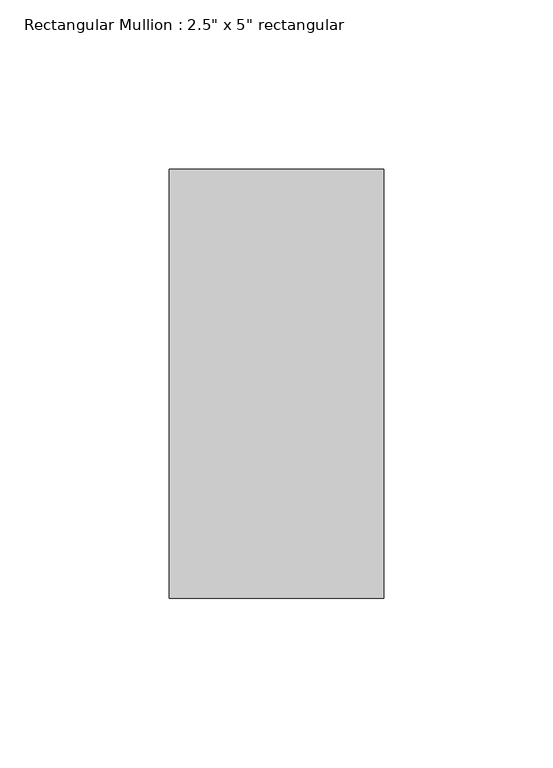
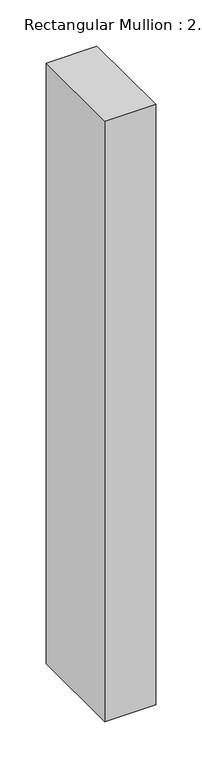
"""IFC4 building model written with IfcOpenShell, lengths in millimetres: member geometry."""

from ifc_helpers import new_model, si_unit, frame, origin, place, context, project, spatial, polyline, outline, extrude, source, transform, mapped, element, save


def member_13dc6413(model_context):
    return source(origin(), model_context, "Body", "SweptSolid", [
        extrude(outline(polyline([(0.0, 63.5), (0.0, -63.5), (-63.5, -63.5), (-63.5, 63.5), (0.0, 63.5)])), frame((0.0, 0.0, -793.75), z_axis=(0.0, 0.0, 1.0), x_axis=(1.0, 0.0, 0.0)), (0.0, 0.0, 1.0), 793.75),
    ])


if __name__ == "__main__":
    model = new_model("IFC4")
    model_context = context("Model", 3, world=origin())
    ifc_project = project(units=[si_unit("LENGTHUNIT", "METRE", prefix="MILLI")], contexts=[model_context])
    site = spatial("IfcSite", under=ifc_project)
    building = spatial("IfcBuilding", under=site)
    placement = place(None, origin())
    member_shape = member_13dc6413(model_context)
    element("IfcMember", 1, ObjectType="Rectangular Mullion : 2.5\" x 5\" rectangular", at=placement, inside=building, context=model_context, shape_type="MappedRepresentation", body=[
        mapped(member_shape, transform((0.0, 0.0, 0.0), x_axis=(1.0, 0.0, 0.0), y_axis=(0.0, 1.0, 0.0), z_axis=(0.0, 0.0, 1.0))),
    ])
    save(model, "model.ifc")

# Revit data of these elements
# Type "Rectangular Mullion : 2.5\" x 5\" rectangular"
#   built-in parameter 1007304 = 0.416667 (stored number, unit not read)
#   built-in parameter 1007301 = 0.104167 (stored number, unit not read)
#   built-in parameter 1007300 = 0.104167 (stored number, unit not read)
# Element 1 (IfcMember, "Rectangular Mullion : 2.5\" x 5\" rectangular")
#   Materials on its faces: "Aluminum"
# Materials
#   "Aluminum": class "Metal", colour RGB 247 247 247, transparency 0, Description = "Aluminum 6061", Cost = 0
